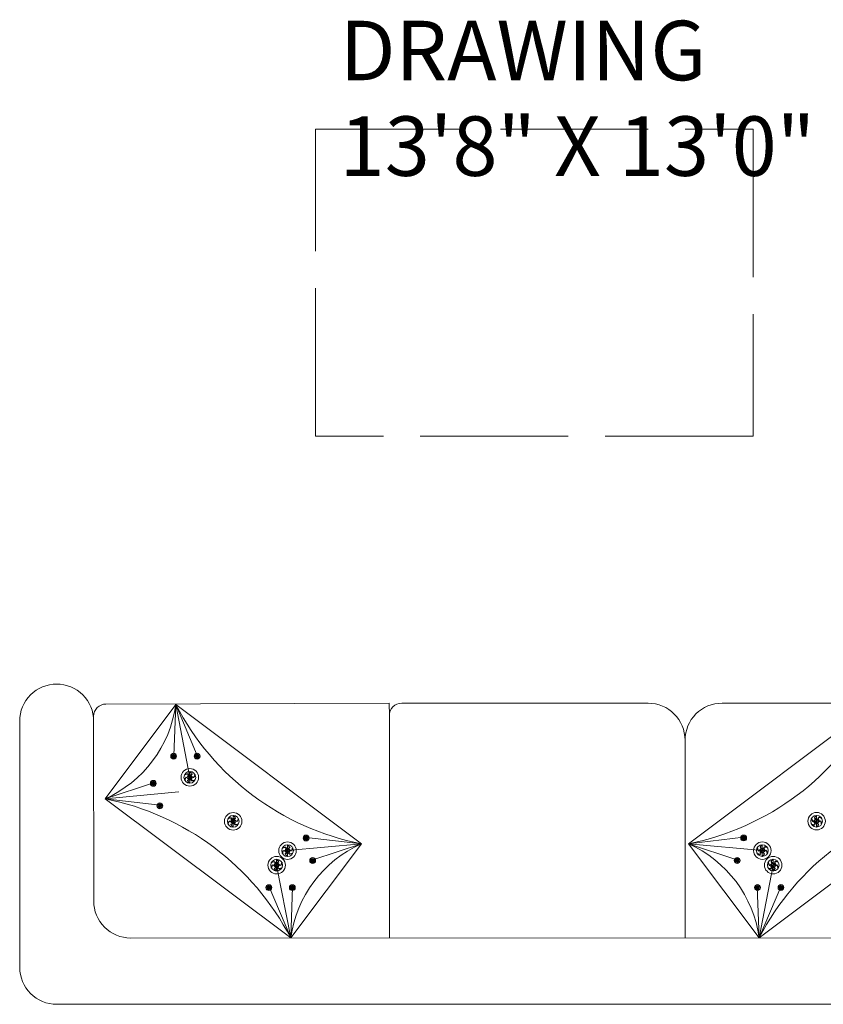
# Model space of a CAD drawing. Units: inches. Extents: x -61 to 1599, y -1316 to 257.
# Tile 177 of 204: x 1397 to 1463, y -934 to -854. Entities that reach past the tile are written whole.
import ezdxf

# ---------------------------------------------------------------- set-up
doc = ezdxf.new("R2010")
doc.units = ezdxf.units.IN
doc.header["$MEASUREMENT"] = 0
doc.linetypes.add('ACAD_ISO02W100', pattern=[15, 12, -3])
for name, color, linetype, lineweight in [('A-AREA-IDEN', 1, 'Continuous', 18), ('A-FURN-LOW', 83, 'ACAD_ISO02W100', 18), ('FURNITURE', 83, 'Continuous', 18)]:
    doc.layers.add(name, color=color, linetype=linetype, lineweight=lineweight)
doc.layers.add('FUR', color=83, linetype='Continuous')
doc.styles.get("Standard").update_dxf_attribs({"font": 'arial.ttf'})

# ---------------------------------------------------------------- blocks, each defined once
blk = doc.blocks.new('*U368')
at = {"layer": 'FUR'}
blk.add_open_spline([(0.005, 0.08), (-0.03, 0.048), (-0.098, -0.015), (0.075, -0.018), (0.024, -0.063), (0.005, -0.08)], degree=3, knots=[0, 0, 0, 0, 0.0954578, 0.1898773, 0.2470677, 0.2470677, 0.2470677, 0.2470677], dxfattribs=at)
blk = doc.blocks.new('*U369')
at = {"layer": 'FUR', "transparency": 16777216}
for p, rotation in [((222.173, -79.977), 60), ((222.312, -79.968), 300), ((222.178, -80.056), 120), ((222.25, -80.092), 180), ((222.317, -80.048), 240)]:
    blk.add_blockref('*U368', p, dxfattribs=dict(at, rotation=rotation))
blk.add_blockref('*U368', (222.24, -79.932), dxfattribs=at)
blk = doc.blocks.new('*U370')
at = {"layer": 'FUR'}
blk.add_open_spline([(0.005, 0.08), (-0.03, 0.048), (-0.098, -0.015), (0.075, -0.018), (0.024, -0.063), (0.005, -0.08)], degree=3, knots=[0, 0, 0, 0, 0.0954578, 0.1898773, 0.2470677, 0.2470677, 0.2470677, 0.2470677], dxfattribs=at)
blk = doc.blocks.new('*U371')
at = {"layer": 'FUR', "transparency": 16777216}
for p, rotation in [((222.173, -79.977), 60), ((222.312, -79.968), 300), ((222.178, -80.056), 120), ((222.25, -80.092), 180), ((222.317, -80.048), 240)]:
    blk.add_blockref('*U370', p, dxfattribs=dict(at, rotation=rotation))
blk.add_blockref('*U370', (222.24, -79.932), dxfattribs=at)
blk = doc.blocks.new('*U364')
at = {"layer": 'FUR'}
blk.add_open_spline([(0.005, 0.08), (-0.03, 0.048), (-0.098, -0.015), (0.075, -0.018), (0.024, -0.063), (0.005, -0.08)], degree=3, knots=[0, 0, 0, 0, 0.0954578, 0.1898773, 0.2470677, 0.2470677, 0.2470677, 0.2470677], dxfattribs=at)
blk = doc.blocks.new('*U365')
at = {"layer": 'FUR', "transparency": 16777216}
for p, rotation in [((222.173, -79.977), 60), ((222.312, -79.968), 300), ((222.178, -80.056), 120), ((222.25, -80.092), 180), ((222.317, -80.048), 240)]:
    blk.add_blockref('*U364', p, dxfattribs=dict(at, rotation=rotation))
blk.add_blockref('*U364', (222.24, -79.932), dxfattribs=at)
blk = doc.blocks.new('*U333')
at = {"layer": 'FUR'}
blk.add_open_spline([(0.015, 0.238), (-0.088, 0.143), (-0.292, -0.045), (0.224, -0.053), (0.072, -0.187), (0.015, -0.238)], degree=3, knots=[0, 0, 0, 0, 0.2846533, 0.5662105, 0.736751, 0.736751, 0.736751, 0.736751], dxfattribs=at)
blk = doc.blocks.new('*U334')
at = {"layer": 'FUR', "transparency": 16777216}
blk.add_blockref('*U333', (662.716, -238.357), dxfattribs=at)
for p, rotation in [((662.929, -238.463), 300), ((662.517, -238.489), 60), ((662.531, -238.727), 120), ((662.745, -238.833), 180), ((662.944, -238.702), 240)]:
    blk.add_blockref('*U333', p, dxfattribs=dict(at, rotation=rotation))
blk = doc.blocks.new('*U366')
at = {"layer": 'FUR'}
blk.add_open_spline([(0.005, 0.08), (-0.03, 0.048), (-0.098, -0.015), (0.075, -0.018), (0.024, -0.063), (0.005, -0.08)], degree=3, knots=[0, 0, 0, 0, 0.0954578, 0.1898773, 0.2470677, 0.2470677, 0.2470677, 0.2470677], dxfattribs=at)
blk = doc.blocks.new('*U367')
at = {"layer": 'FUR', "transparency": 16777216}
for p, rotation in [((222.173, -79.977), 60), ((222.312, -79.968), 300), ((222.178, -80.056), 120), ((222.25, -80.092), 180), ((222.317, -80.048), 240)]:
    blk.add_blockref('*U366', p, dxfattribs=dict(at, rotation=rotation))
blk.add_blockref('*U366', (222.24, -79.932), dxfattribs=at)
blk = doc.blocks.new('*U337')
at = {"layer": 'FUR'}
blk.add_open_spline([(0.015, 0.238), (-0.088, 0.143), (-0.292, -0.045), (0.224, -0.053), (0.072, -0.187), (0.015, -0.238)], degree=3, knots=[0, 0, 0, 0, 0.2846533, 0.5662105, 0.736751, 0.736751, 0.736751, 0.736751], dxfattribs=at)
blk = doc.blocks.new('*U338')
at = {"layer": 'FUR', "transparency": 16777216}
blk.add_blockref('*U337', (662.716, -238.357), dxfattribs=at)
for p, rotation in [((662.929, -238.463), 300), ((662.517, -238.489), 60), ((662.531, -238.727), 120), ((662.745, -238.833), 180), ((662.944, -238.702), 240)]:
    blk.add_blockref('*U337', p, dxfattribs=dict(at, rotation=rotation))
blk = doc.blocks.new('*U352')
at = {"layer": 'FUR'}
blk.add_open_spline([(0.005, 0.08), (-0.03, 0.048), (-0.098, -0.015), (0.075, -0.018), (0.024, -0.063), (0.005, -0.08)], degree=3, knots=[0, 0, 0, 0, 0.0954578, 0.1898773, 0.2470677, 0.2470677, 0.2470677, 0.2470677], dxfattribs=at)
blk = doc.blocks.new('*U353')
at = {"layer": 'FUR', "transparency": 16777216}
for p, rotation in [((222.173, -79.977), 60), ((222.312, -79.968), 300), ((222.178, -80.056), 120), ((222.25, -80.092), 180), ((222.317, -80.048), 240)]:
    blk.add_blockref('*U352', p, dxfattribs=dict(at, rotation=rotation))
blk.add_blockref('*U352', (222.24, -79.932), dxfattribs=at)
blk = doc.blocks.new('*U339')
at = {"layer": 'FUR'}
blk.add_open_spline([(0.015, 0.238), (-0.088, 0.143), (-0.292, -0.045), (0.224, -0.053), (0.072, -0.187), (0.015, -0.238)], degree=3, knots=[0, 0, 0, 0, 0.2846533, 0.5662105, 0.736751, 0.736751, 0.736751, 0.736751], dxfattribs=at)
blk = doc.blocks.new('*U351')
at = {"layer": 'FUR', "transparency": 16777216}
blk.add_blockref('*U339', (662.716, -238.357), dxfattribs=at)
for p, rotation in [((662.929, -238.463), 300), ((662.517, -238.489), 60), ((662.531, -238.727), 120), ((662.745, -238.833), 180), ((662.944, -238.702), 240)]:
    blk.add_blockref('*U339', p, dxfattribs=dict(at, rotation=rotation))
blk = doc.blocks.new('*U335')
at = {"layer": 'FUR'}
blk.add_open_spline([(0.015, 0.238), (-0.088, 0.143), (-0.292, -0.045), (0.224, -0.053), (0.072, -0.187), (0.015, -0.238)], degree=3, knots=[0, 0, 0, 0, 0.2846533, 0.5662105, 0.736751, 0.736751, 0.736751, 0.736751], dxfattribs=at)
blk = doc.blocks.new('*U336')
at = {"layer": 'FUR', "transparency": 16777216}
blk.add_blockref('*U335', (662.716, -238.357), dxfattribs=at)
for p, rotation in [((662.929, -238.463), 300), ((662.517, -238.489), 60), ((662.531, -238.727), 120), ((662.745, -238.833), 180), ((662.944, -238.702), 240)]:
    blk.add_blockref('*U335', p, dxfattribs=dict(at, rotation=rotation))
blk = doc.blocks.new('*U331')
at = {"layer": 'FUR'}
blk.add_open_spline([(0.005, 0.08), (-0.03, 0.048), (-0.098, -0.015), (0.075, -0.018), (0.024, -0.063), (0.005, -0.08)], degree=3, knots=[0, 0, 0, 0, 0.0954578, 0.1898773, 0.2470677, 0.2470677, 0.2470677, 0.2470677], dxfattribs=at)
blk = doc.blocks.new('*U332')
at = {"layer": 'FUR', "transparency": 16777216}
for p, rotation in [((222.173, -79.977), 60), ((222.312, -79.968), 300), ((222.178, -80.056), 120), ((222.25, -80.092), 180), ((222.317, -80.048), 240)]:
    blk.add_blockref('*U331', p, dxfattribs=dict(at, rotation=rotation))
blk.add_blockref('*U331', (222.24, -79.932), dxfattribs=at)
blk = doc.blocks.new('*U362')
at = {"layer": 'FUR'}
blk.add_open_spline([(0.005, 0.08), (-0.03, 0.048), (-0.098, -0.015), (0.075, -0.018), (0.024, -0.063), (0.005, -0.08)], degree=3, knots=[0, 0, 0, 0, 0.0954578, 0.1898773, 0.2470677, 0.2470677, 0.2470677, 0.2470677], dxfattribs=at)
blk = doc.blocks.new('*U363')
at = {"layer": 'FUR', "transparency": 16777216}
for p, rotation in [((222.173, -79.977), 60), ((222.312, -79.968), 300), ((222.178, -80.056), 120), ((222.25, -80.092), 180), ((222.317, -80.048), 240)]:
    blk.add_blockref('*U362', p, dxfattribs=dict(at, rotation=rotation))
blk.add_blockref('*U362', (222.24, -79.932), dxfattribs=at)
blk = doc.blocks.new('*U360')
at = {"layer": 'FUR'}
blk.add_open_spline([(0.005, 0.08), (-0.03, 0.048), (-0.098, -0.015), (0.075, -0.018), (0.024, -0.063), (0.005, -0.08)], degree=3, knots=[0, 0, 0, 0, 0.0954578, 0.1898773, 0.2470677, 0.2470677, 0.2470677, 0.2470677], dxfattribs=at)
blk = doc.blocks.new('*U361')
at = {"layer": 'FUR', "transparency": 16777216}
for p, rotation in [((222.173, -79.977), 60), ((222.312, -79.968), 300), ((222.178, -80.056), 120), ((222.25, -80.092), 180), ((222.317, -80.048), 240)]:
    blk.add_blockref('*U360', p, dxfattribs=dict(at, rotation=rotation))
blk.add_blockref('*U360', (222.24, -79.932), dxfattribs=at)
blk = doc.blocks.new('*U330')
at = {"layer": 'FUR'}
blk.add_open_spline([(0.005, 0.08), (-0.03, 0.048), (-0.098, -0.015), (0.075, -0.018), (0.024, -0.063), (0.005, -0.08)], degree=3, knots=[0, 0, 0, 0, 0.0954578, 0.1898773, 0.2470677, 0.2470677, 0.2470677, 0.2470677], dxfattribs=at)
blk = doc.blocks.new('*U343')
at = {"layer": 'FUR', "transparency": 16777216}
for p, rotation in [((222.173, -79.977), 60), ((222.312, -79.968), 300), ((222.178, -80.056), 120), ((222.25, -80.092), 180), ((222.317, -80.048), 240)]:
    blk.add_blockref('*U330', p, dxfattribs=dict(at, rotation=rotation))
blk.add_blockref('*U330', (222.24, -79.932), dxfattribs=at)
blk = doc.blocks.new('*U344')
at = {"layer": 'FUR'}
blk.add_open_spline([(0.005, 0.08), (-0.03, 0.048), (-0.098, -0.015), (0.075, -0.018), (0.024, -0.063), (0.005, -0.08)], degree=3, knots=[0, 0, 0, 0, 0.0954578, 0.1898773, 0.2470677, 0.2470677, 0.2470677, 0.2470677], dxfattribs=at)
blk = doc.blocks.new('*U345')
at = {"layer": 'FUR', "transparency": 16777216}
for p, rotation in [((222.173, -79.977), 60), ((222.312, -79.968), 300), ((222.178, -80.056), 120), ((222.25, -80.092), 180), ((222.317, -80.048), 240)]:
    blk.add_blockref('*U344', p, dxfattribs=dict(at, rotation=rotation))
blk.add_blockref('*U344', (222.24, -79.932), dxfattribs=at)
blk = doc.blocks.new('*U328')
at = {"layer": 'FUR'}
blk.add_open_spline([(0.005, 0.08), (-0.03, 0.048), (-0.098, -0.015), (0.075, -0.018), (0.024, -0.063), (0.005, -0.08)], degree=3, knots=[0, 0, 0, 0, 0.0954578, 0.1898773, 0.2470677, 0.2470677, 0.2470677, 0.2470677], dxfattribs=at)
blk = doc.blocks.new('*U329')
at = {"layer": 'FUR', "transparency": 16777216}
for p, rotation in [((222.173, -79.977), 60), ((222.312, -79.968), 300), ((222.178, -80.056), 120), ((222.25, -80.092), 180), ((222.317, -80.048), 240)]:
    blk.add_blockref('*U328', p, dxfattribs=dict(at, rotation=rotation))
blk.add_blockref('*U328', (222.24, -79.932), dxfattribs=at)
blk = doc.blocks.new('*U358')
at = {"layer": 'FUR'}
blk.add_open_spline([(0.015, 0.238), (-0.088, 0.143), (-0.292, -0.045), (0.224, -0.053), (0.072, -0.187), (0.015, -0.238)], degree=3, knots=[0, 0, 0, 0, 0.2846533, 0.5662105, 0.736751, 0.736751, 0.736751, 0.736751], dxfattribs=at)
blk = doc.blocks.new('*U359')
at = {"layer": 'FUR', "transparency": 16777216}
blk.add_blockref('*U358', (662.716, -238.357), dxfattribs=at)
for p, rotation in [((662.929, -238.463), 300), ((662.517, -238.489), 60), ((662.531, -238.727), 120), ((662.745, -238.833), 180), ((662.944, -238.702), 240)]:
    blk.add_blockref('*U358', p, dxfattribs=dict(at, rotation=rotation))
blk = doc.blocks.new('*U374')
at = {"layer": 'FUR'}
blk.add_open_spline([(0.015, 0.238), (-0.088, 0.143), (-0.292, -0.045), (0.224, -0.053), (0.072, -0.187), (0.015, -0.238)], degree=3, knots=[0, 0, 0, 0, 0.2846533, 0.5662105, 0.736751, 0.736751, 0.736751, 0.736751], dxfattribs=at)
blk = doc.blocks.new('*U325')
at = {"layer": 'FUR', "transparency": 16777216}
blk.add_blockref('*U374', (662.716, -238.357), dxfattribs=at)
for p, rotation in [((662.929, -238.463), 300), ((662.517, -238.489), 60), ((662.531, -238.727), 120), ((662.745, -238.833), 180), ((662.944, -238.702), 240)]:
    blk.add_blockref('*U374', p, dxfattribs=dict(at, rotation=rotation))
blk = doc.blocks.new('*U326')
at = {"layer": 'FUR'}
blk.add_open_spline([(0.005, 0.08), (-0.03, 0.048), (-0.098, -0.015), (0.075, -0.018), (0.024, -0.063), (0.005, -0.08)], degree=3, knots=[0, 0, 0, 0, 0.0954578, 0.1898773, 0.2470677, 0.2470677, 0.2470677, 0.2470677], dxfattribs=at)
blk = doc.blocks.new('*U327')
at = {"layer": 'FUR', "transparency": 16777216}
for p, rotation in [((222.173, -79.977), 60), ((222.312, -79.968), 300), ((222.178, -80.056), 120), ((222.25, -80.092), 180), ((222.317, -80.048), 240)]:
    blk.add_blockref('*U326', p, dxfattribs=dict(at, rotation=rotation))
blk.add_blockref('*U326', (222.24, -79.932), dxfattribs=at)
blk = doc.blocks.new('*U372')
at = {"layer": 'FUR'}
blk.add_open_spline([(0.015, 0.238), (-0.088, 0.143), (-0.292, -0.045), (0.224, -0.053), (0.072, -0.187), (0.015, -0.238)], degree=3, knots=[0, 0, 0, 0, 0.2846533, 0.5662105, 0.736751, 0.736751, 0.736751, 0.736751], dxfattribs=at)
blk = doc.blocks.new('*U373')
at = {"layer": 'FUR', "transparency": 16777216}
blk.add_blockref('*U372', (662.716, -238.357), dxfattribs=at)
for p, rotation in [((662.929, -238.463), 300), ((662.517, -238.489), 60), ((662.531, -238.727), 120), ((662.745, -238.833), 180), ((662.944, -238.702), 240)]:
    blk.add_blockref('*U372', p, dxfattribs=dict(at, rotation=rotation))
blk = doc.blocks.new('*U348')
at = {"layer": 'FUR'}
blk.add_open_spline([(0.005, 0.08), (-0.03, 0.048), (-0.098, -0.015), (0.075, -0.018), (0.024, -0.063), (0.005, -0.08)], degree=3, knots=[0, 0, 0, 0, 0.0954578, 0.1898773, 0.2470677, 0.2470677, 0.2470677, 0.2470677], dxfattribs=at)
blk = doc.blocks.new('*U349')
at = {"layer": 'FUR', "transparency": 16777216}
for p, rotation in [((222.173, -79.977), 60), ((222.312, -79.968), 300), ((222.178, -80.056), 120), ((222.25, -80.092), 180), ((222.317, -80.048), 240)]:
    blk.add_blockref('*U348', p, dxfattribs=dict(at, rotation=rotation))
blk.add_blockref('*U348', (222.24, -79.932), dxfattribs=at)
blk = doc.blocks.new('*U356')
at = {"layer": 'FUR'}
blk.add_open_spline([(0.015, 0.238), (-0.088, 0.143), (-0.292, -0.045), (0.224, -0.053), (0.072, -0.187), (0.015, -0.238)], degree=3, knots=[0, 0, 0, 0, 0.2846533, 0.5662105, 0.736751, 0.736751, 0.736751, 0.736751], dxfattribs=at)
blk = doc.blocks.new('*U357')
at = {"layer": 'FUR', "transparency": 16777216}
blk.add_blockref('*U356', (662.716, -238.357), dxfattribs=at)
for p, rotation in [((662.929, -238.463), 300), ((662.517, -238.489), 60), ((662.531, -238.727), 120), ((662.745, -238.833), 180), ((662.944, -238.702), 240)]:
    blk.add_blockref('*U356', p, dxfattribs=dict(at, rotation=rotation))
blk = doc.blocks.new('*U340')
at = {"layer": 'FUR'}
blk.add_open_spline([(0.015, 0.238), (-0.088, 0.143), (-0.292, -0.045), (0.224, -0.053), (0.072, -0.187), (0.015, -0.238)], degree=3, knots=[0, 0, 0, 0, 0.2846533, 0.5662105, 0.736751, 0.736751, 0.736751, 0.736751], dxfattribs=at)
blk = doc.blocks.new('*U341')
at = {"layer": 'FUR', "transparency": 16777216}
blk.add_blockref('*U340', (662.716, -238.357), dxfattribs=at)
for p, rotation in [((662.929, -238.463), 300), ((662.517, -238.489), 60), ((662.531, -238.727), 120), ((662.745, -238.833), 180), ((662.944, -238.702), 240)]:
    blk.add_blockref('*U340', p, dxfattribs=dict(at, rotation=rotation))
blk = doc.blocks.new('*U346')
at = {"layer": 'FUR'}
blk.add_open_spline([(0.005, 0.08), (-0.03, 0.048), (-0.098, -0.015), (0.075, -0.018), (0.024, -0.063), (0.005, -0.08)], degree=3, knots=[0, 0, 0, 0, 0.0954578, 0.1898773, 0.2470677, 0.2470677, 0.2470677, 0.2470677], dxfattribs=at)
blk = doc.blocks.new('*U347')
at = {"layer": 'FUR', "transparency": 16777216}
for p, rotation in [((222.173, -79.977), 60), ((222.312, -79.968), 300), ((222.178, -80.056), 120), ((222.25, -80.092), 180), ((222.317, -80.048), 240)]:
    blk.add_blockref('*U346', p, dxfattribs=dict(at, rotation=rotation))
blk.add_blockref('*U346', (222.24, -79.932), dxfattribs=at)
blk = doc.blocks.new('*U354')
at = {"layer": 'FUR'}
blk.add_open_spline([(0.005, 0.08), (-0.03, 0.048), (-0.098, -0.015), (0.075, -0.018), (0.024, -0.063), (0.005, -0.08)], degree=3, knots=[0, 0, 0, 0, 0.0954578, 0.1898773, 0.2470677, 0.2470677, 0.2470677, 0.2470677], dxfattribs=at)
blk = doc.blocks.new('*U355')
at = {"layer": 'FUR', "transparency": 16777216}
for p, rotation in [((222.173, -79.977), 60), ((222.312, -79.968), 300), ((222.178, -80.056), 120), ((222.25, -80.092), 180), ((222.317, -80.048), 240)]:
    blk.add_blockref('*U354', p, dxfattribs=dict(at, rotation=rotation))
blk.add_blockref('*U354', (222.24, -79.932), dxfattribs=at)
blk = doc.blocks.new('*U350')
at = {"layer": 'FUR'}
blk.add_open_spline([(0.005, 0.08), (-0.03, 0.048), (-0.098, -0.015), (0.075, -0.018), (0.024, -0.063), (0.005, -0.08)], degree=3, knots=[0, 0, 0, 0, 0.0954578, 0.1898773, 0.2470677, 0.2470677, 0.2470677, 0.2470677], dxfattribs=at)
blk = doc.blocks.new('*U342')
at = {"layer": 'FUR', "transparency": 16777216}
for p, rotation in [((222.173, -79.977), 60), ((222.312, -79.968), 300), ((222.178, -80.056), 120), ((222.25, -80.092), 180), ((222.317, -80.048), 240)]:
    blk.add_blockref('*U350', p, dxfattribs=dict(at, rotation=rotation))
blk.add_blockref('*U350', (222.24, -79.932), dxfattribs=at)
blk = doc.blocks.new('SOFA-THREE-SEAT-ALT')
for p, q in [((30, 24.442), (6.996, 24.38)), ((12.664, 24.334), (12.509, 20.192)), ((12.664, 24.334), (13.805, 18.423)), ((12.664, 24.334), (14.414, 20.192)), ((30, 23.442), (29.997, 24.442)), ((51, 24.442), (31, 24.442)), ((78.369, 24.442), (57, 24.442)), ((69.336, 24.334), (67.586, 20.192)), ((69.336, 24.334), (68.194, 18.423)), ((69.336, 24.334), (69.49, 20.192)), ((6, 23), (5.999, 23.378)), ((30, 23.442), (30, 5.382)), ((54, 21.442), (54, 5.382)), ((54, 21.442), (54, 21.442)), ((12.49, 20.139), (12.49, 20.299)), ((12.49, 20.139), (12.49, 19.98)), ((14.394, 20.139), (14.394, 20.299)), ((14.394, 20.139), (14.394, 19.98)), ((67.605, 20.139), (67.605, 20.299)), ((67.605, 20.139), (67.605, 19.98)), ((69.509, 20.139), (69.509, 20.299)), ((69.509, 20.139), (69.509, 19.98)), ((13.805, 18.423), (13.805, 18.9)), ((13.805, 18.423), (13.805, 17.947)), ((68.194, 18.423), (68.194, 18.9)), ((68.194, 18.423), (68.194, 17.947)), ((6.926, 16.688), (10.859, 17.993)), ((10.84, 17.94), (10.84, 18.1)), ((10.84, 17.94), (10.84, 17.781)), ((69.079, 17.243), (69.079, 17.72)), ((75.074, 16.688), (71.14, 17.993)), ((71.159, 17.94), (71.159, 18.1)), ((71.159, 17.94), (71.159, 17.781)), ((6.926, 16.688), (12.92, 17.243)), ((75.074, 16.688), (69.079, 17.243)), ((69.079, 17.243), (69.079, 16.767)), ((6.926, 16.688), (11.391, 16.165)), ((11.372, 16.112), (11.372, 16.272)), ((11.372, 16.112), (11.372, 15.952)), ((75.074, 16.688), (70.608, 16.165)), ((70.627, 16.112), (70.627, 16.272)), ((70.627, 16.112), (70.627, 15.952)), ((17.327, 14.858), (17.327, 15.334)), ((64.672, 14.858), (64.672, 15.334)), ((17.327, 14.858), (17.327, 14.381)), ((64.672, 14.858), (64.672, 14.381)), ((23.243, 13.498), (23.243, 13.658)), ((58.756, 13.498), (58.756, 13.658)), ((27.729, 13.028), (21.735, 12.472)), ((21.735, 12.472), (21.735, 12.949)), ((23.243, 13.498), (23.243, 13.339)), ((27.729, 13.028), (23.263, 13.551)), ((27.729, 13.028), (23.795, 11.723)), ((54.271, 13.028), (58.736, 13.551)), ((54.271, 13.028), (60.265, 12.472)), ((54.271, 13.028), (58.204, 11.723)), ((58.756, 13.498), (58.756, 13.339)), ((60.265, 12.472), (60.265, 12.949)), ((21.735, 12.472), (21.735, 11.996)), ((60.265, 12.472), (60.265, 11.996)), ((20.849, 11.293), (20.849, 11.769)), ((21.991, 5.382), (20.849, 11.293)), ((20.849, 11.293), (20.849, 10.816)), ((23.776, 11.67), (23.776, 11.83)), ((23.776, 11.67), (23.776, 11.51)), ((58.224, 11.67), (58.224, 11.83)), ((58.224, 11.67), (58.224, 11.51)), ((60.009, 5.382), (61.15, 11.293)), ((61.15, 11.293), (61.15, 11.769)), ((61.15, 11.293), (61.15, 10.816)), ((20.221, 9.471), (20.221, 9.631)), ((22.125, 9.471), (22.125, 9.631)), ((59.874, 9.471), (59.874, 9.631)), ((61.778, 9.471), (61.778, 9.631)), ((20.221, 9.471), (20.221, 9.311)), ((21.991, 5.382), (20.241, 9.524)), ((21.991, 5.382), (22.145, 9.524)), ((22.125, 9.471), (22.125, 9.311)), ((60.009, 5.382), (59.854, 9.524)), ((59.874, 9.471), (59.874, 9.311)), ((60.009, 5.382), (61.759, 9.524)), ((61.778, 9.471), (61.778, 9.311))]:
    blk.add_line(p, q)
blk.add_lwpolyline([(78, 8.382), (78, 23, -0.414214), (81, 26), (81, 26, -0.414214), (84, 23), (84, 3, -0.414214), (81, 0), (3, 0, -0.414214), (0, 3), (0, 23, -0.414214), (3, 26), (3, 26, -0.414214), (6, 23), (6, 8.382, 0.414214), (9, 5.382), (75, 5.382, 0.414214)], format="xyb", close=True)
for points in [[(27.729, 13.028), (12.664, 24.334), (6.926, 16.688), (21.991, 5.382)], [(54.271, 13.028), (69.336, 24.334), (75.074, 16.688), (60.009, 5.382)]]:
    blk.add_lwpolyline(points, close=True)
for centre, radius in [((12.49, 20.139), 0.238), ((12.49, 20.139), 0.16), ((14.394, 20.139), 0.238), ((14.394, 20.139), 0.16), ((67.605, 20.139), 0.238), ((67.605, 20.139), 0.16), ((69.509, 20.139), 0.238), ((69.509, 20.139), 0.16), ((13.805, 18.423), 0.71), ((13.805, 18.423), 0.476), ((68.194, 18.423), 0.71), ((68.194, 18.423), 0.476), ((10.84, 17.94), 0.238), ((10.84, 17.94), 0.16), ((69.079, 17.243), 0.71), ((69.079, 17.243), 0.476), ((71.159, 17.94), 0.238), ((71.159, 17.94), 0.16), ((11.372, 16.112), 0.238), ((11.372, 16.112), 0.16), ((70.627, 16.112), 0.238), ((70.627, 16.112), 0.16), ((17.327, 14.858), 0.71), ((17.327, 14.858), 0.476), ((64.672, 14.858), 0.71), ((64.672, 14.858), 0.476), ((23.243, 13.498), 0.238), ((23.243, 13.498), 0.16), ((58.756, 13.498), 0.238), ((58.756, 13.498), 0.16), ((21.735, 12.472), 0.71), ((21.735, 12.472), 0.476), ((60.265, 12.472), 0.71), ((60.265, 12.472), 0.476), ((20.849, 11.293), 0.71), ((61.15, 11.293), 0.71), ((20.849, 11.293), 0.476), ((23.776, 11.67), 0.238), ((23.776, 11.67), 0.16), ((58.224, 11.67), 0.238), ((58.224, 11.67), 0.16), ((61.15, 11.293), 0.476), ((20.221, 9.471), 0.238), ((20.221, 9.471), 0.16), ((22.125, 9.471), 0.238), ((22.125, 9.471), 0.16), ((59.874, 9.471), 0.238), ((59.874, 9.471), 0.16), ((61.778, 9.471), 0.238), ((61.778, 9.471), 0.16)]:
    blk.add_circle(centre, radius)
for centre, radius, start, end in [((6.999, 23.38), 1, 90.15417, 180.15417), ((2.937, 25.657), 9.816, 293.97422, 352.25297), ((31.951, 34.345), 21.731, 207.43163, 258.79556), ((31, 23.442), 1, 89.99998, 179.99998), ((51, 21.442), 3, 359.99998, 89.99998), ((57, 21.442), 3, 90, 180.00002), ((50.048, 34.345), 21.731, 281.20444, 332.56837), ((79.062, 25.657), 9.816, 187.74703, 246.02578), ((2.703, -4.629), 21.731, 27.43163, 78.79556), ((79.296, -4.629), 21.731, 101.20444, 152.56837), ((31.717, 4.059), 9.816, 113.97422, 172.25297), ((50.282, 4.059), 9.816, 7.74703, 66.02578)]:
    blk.add_arc(centre, radius, start, end)
at = {"xscale": -1, "rotation": 180}
for name, p in [('*U365', (-209.755, -59.873)), ('*U367', (-207.851, -59.873)), ('*U334', (-648.925, -220.172)), ('*U369', (-211.405, -62.072)), ('*U371', (-210.873, -63.9)), ('*U338', (-645.403, -223.737)), ('*U363', (-199.001, -66.514)), ('*U336', (-640.996, -226.123)), ('*U351', (-641.881, -227.303)), ('*U361', (-198.469, -68.342)), ('*U353', (-202.024, -70.541)), ('*U332', (-200.12, -70.541))]:
    blk.add_blockref(name, p, dxfattribs=at)
at = {"rotation": 180}
for name, p in [('*U349', (289.85, -59.873)), ('*U347', (291.754, -59.873)), ('*U357', (730.924, -220.172)), ('*U341', (731.81, -221.352)), ('*U342', (293.404, -62.072)), ('*U355', (292.872, -63.9)), ('*U373', (727.402, -223.737)), ('*U345', (281.001, -66.514)), ('*U359', (722.995, -226.123)), ('*U343', (280.469, -68.342)), ('*U325', (723.88, -227.303)), ('*U329', (282.119, -70.541)), ('*U327', (284.023, -70.541))]:
    blk.add_blockref(name, p, dxfattribs=at)

msp = doc.modelspace()

# ---------------------------------------------------------------- linework, layer by layer
at = {"layer": 'A-FURN-LOW'}
msp.add_lwpolyline([(1456.9662, -887.802), (1421.4644, -887.802), (1421.4644, -862.8983), (1456.9662, -862.8983)], close=True, dxfattribs=at)

# ---------------------------------------------------------------- block references
at = {"layer": 'FURNITURE', "rotation": 0.0082401218147832}
msp.add_blockref('SOFA-THREE-SEAT-ALT', (1397.4562, -933.9417), dxfattribs=at)

# ---------------------------------------------------------------- texts
at = {"layer": 'A-AREA-IDEN'}
for s, height, p in [('DRAWING', 4.8321, (1423.4206, -858.9153)), ('13\'8" X 13\'0"', 4.832098, (1423.4206, -866.6776))]:
    msp.add_text(s, height=height, dxfattribs=at).set_placement(p)

doc.saveas('drawing.dxf')
